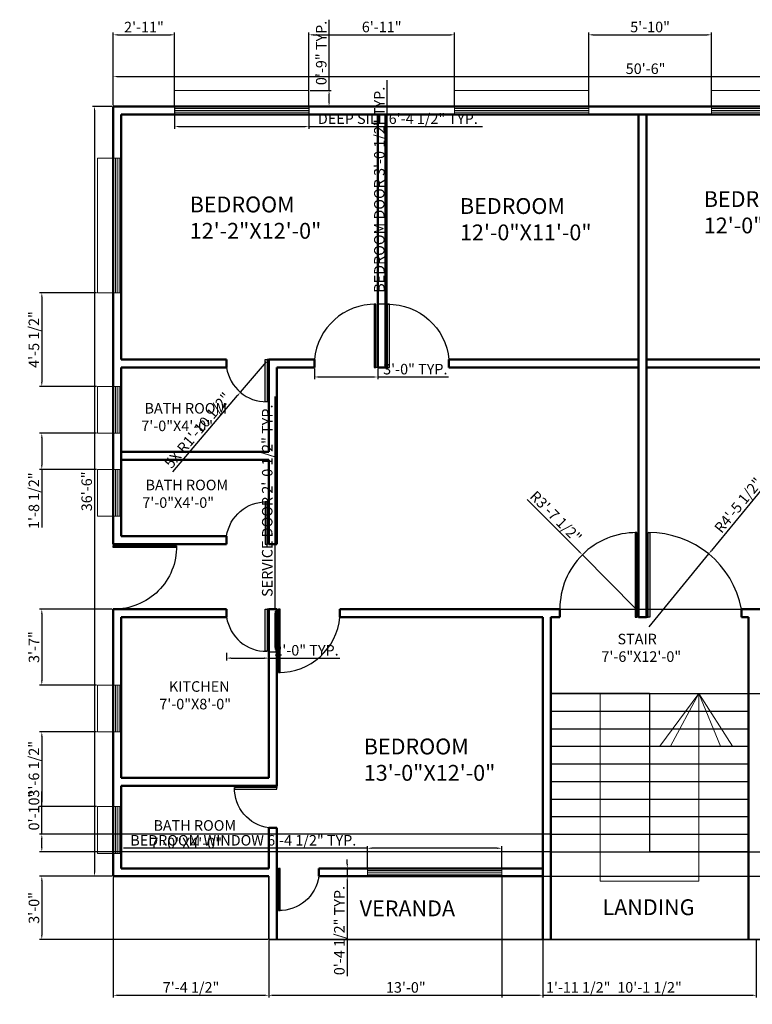
# Model space of a CAD drawing. Units: inches. Extents: x 2373 to 3112, y 1710 to 2270.
# Tile 1 of 2: x 2373 to 2790, y 1710 to 2270. Entities that reach past the tile are written whole.
import ezdxf

# ---------------------------------------------------------------- set-up
doc = ezdxf.new("R2010")
doc.units = ezdxf.units.IN
doc.layers.add('A-ANNO-DIMS', color=7, linetype='Continuous', lineweight=18)
doc.layers.add('A-AREA-IDEN', color=7, linetype='Continuous', lineweight=25)
for name, color, linetype, lineweight, true_color in [('A-ANNO-SYMB', 12, 'Continuous', 18, 0xbc0111), ('A-DOOR', 114, 'Continuous', 25, 0x139b48), ('A-FLOR', 114, 'Continuous', 35, 0x139b48), ('A-FLOR-STRS', 114, 'Continuous', 25, 0x139b48), ('A-GLAZ', 31, 'Continuous', 18, 0xfecc66), ('A-GLAZ-SILL', 30, 'Continuous', 18, 0xf8991e), ('A-WALL', 114, 'Continuous', 50, 0x139b48)]:
    doc.layers.add(name, color=color, linetype=linetype, lineweight=lineweight, true_color=true_color)
doc.styles.get("Standard").update_dxf_attribs({"font": 'arial.ttf'})
doc.dimstyles.new('ISO-25', dxfattribs={"dimtxt": 6, "dimasz": 2.5, "dimexe": 1.25, "dimexo": 0.625, "dimtad": 1, "dimdec": 1, "dimlunit": 3, "dimtxsty": 'Standard', "dimcen": 2.5, "dimadec": 0, "dimazin": 0, "dimtfac": 1, "dimtdec": 1, "dimtmove": 0, "dimatfit": 3, "dimfxl": 1, "dimarcsym": 0})

# ---------------------------------------------------------------- blocks, each defined once
blk = doc.blocks.new('*D2')
at = {"layer": 'A-ANNO-DIMS', "color": 0, "lineweight": -2, "transparency": 16777216}
for p, q in [((2426.36, 2221.72), (2426.36, 2239.32)), ((2428.86, 2238.07), (3029.86, 2238.07)), ((3032.36, 2221.72), (3032.36, 2239.32))]:
    blk.add_line(p, q, dxfattribs=at)
at = {"layer": 'A-ANNO-DIMS', "color": 0, "transparency": 16777216}
for points in [[(2428.86, 2238.48), (2428.86, 2237.65), (2426.36, 2238.07)], [(3029.86, 2238.48), (3029.86, 2237.65), (3032.36, 2238.07)]]:
    blk.add_solid(points, dxfattribs=at)
at = {"layer": 'Defpoints', "color": 0, "transparency": 16777216}
for p in [(3032.36, 2238.07), (2426.36, 2221.09), (3032.36, 2221.09)]:
    blk.add_point(p, dxfattribs=at)
at = {"layer": 'A-ANNO-DIMS', "color": 0, "transparency": 16777216, "insert": (2729.36, 2241.76), "char_height": 6, "attachment_point": 5}
blk.add_mtext('50\'-6"', dxfattribs=at)
blk = doc.blocks.new('*D3')
at = {"layer": 'A-ANNO-DIMS', "color": 0, "lineweight": -2, "transparency": 16777216}
for p, q in [((2425.74, 2221.09), (2414.44, 2221.09)), ((2415.69, 2218.59), (2415.69, 1785.59)), ((2425.74, 1783.09), (2414.44, 1783.09))]:
    blk.add_line(p, q, dxfattribs=at)
at = {"layer": 'A-ANNO-DIMS', "color": 0, "transparency": 16777216}
for points in [[(2415.27, 2218.59), (2416.11, 2218.59), (2415.69, 2221.09)], [(2415.27, 1785.59), (2416.11, 1785.59), (2415.69, 1783.09)]]:
    blk.add_solid(points, dxfattribs=at)
at = {"layer": 'Defpoints', "color": 0, "transparency": 16777216}
for p in [(2426.36, 2221.09), (2415.69, 1783.09), (2426.36, 1783.09)]:
    blk.add_point(p, dxfattribs=at)
at = {"layer": 'A-ANNO-DIMS', "color": 0, "transparency": 16777216, "insert": (2412, 2002.09), "char_height": 6, "attachment_point": 5, "rotation": 90}
blk.add_mtext('36\'-6"', dxfattribs=at)
blk = doc.blocks.new('DOOR-SWING-24IN')
for p, q in [((-2, -24), (-2, 0)), ((-2, 0), (-1, 0)), ((0, 0), (-1, 0)), ((-1, 0), (-1, -24)), ((-1, -24), (-2, -24))]:
    blk.add_line(p, q)
blk.add_arc((-1.5, -1.28), 22.73, 188.1552, 271.2605)
blk = doc.blocks.new('DOOR-SWING-36IN')
for p, q in [((-1, 36), (-2, 36)), ((-2, 36), (-2, 0)), ((-1, 0), (-1, 36)), ((-2, 0), (-1, 0)), ((0, 0), (-1, 0))]:
    blk.add_line(p, q)
blk.add_arc((-1.5, 1.36), 34.64, 89.173, 174.8014)
blk = doc.blocks.new('DOOR-SIDE-ENTRY-36IN')
for p, q in [((0, 0), (0, -1)), ((0, -1), (-36, -1)), ((-36, -1), (-36, -2)), ((-36, -2), (0, -2)), ((0, -2), (0, -1))]:
    blk.add_line(p, q)
blk.add_arc((-0.5, -1.5), 35.5, 179.1931, 270.8069)
blk = doc.blocks.new('WINDOW-BEDROOM')
for p, q in [((0, 0), (0, -4.5)), ((76.46, 0), (0, 0)), ((0, 0), (0, -2.25)), ((76.46, -4.5), (76.46, 0)), ((76.46, -1.25), (0, -1.25)), ((0, -1.25), (0, -2.25)), ((0, -2.25), (76.46, -2.25)), ((0, -2.25), (0, -3.25)), ((0, -3.25), (76.46, -3.25)), ((0, -4.5), (76.46, -4.5)), ((76.46, -2.25), (76.46, -1.25))]:
    blk.add_line(p, q)
blk = doc.blocks.new('WINDOW-SERVICE')
for p, q in [((0, 0), (0, -26.66)), ((4.5, 0), (0, 0)), ((1.25, 0), (1.25, -26.66)), ((2.25, 0), (2.25, -26.66)), ((3.25, -26.66), (3.25, 0)), ((4.5, -26.66), (4.5, 0)), ((4.5, -26.66), (4.5, 0)), ((0, -26.66), (4.5, -26.66))]:
    blk.add_line(p, q)
blk = doc.blocks.new('SILL-SERVICE')
for p, q in [((0, 0), (9, 0)), ((9, 0), (9, -26.66)), ((9, -26.66), (0, -26.66))]:
    blk.add_line(p, q)
blk = doc.blocks.new('SILL-BEDROOM')
for p, q in [((0, 0), (0, 9)), ((0, 9), (76.46, 9)), ((76.46, 9), (76.46, 0))]:
    blk.add_line(p, q)
blk = doc.blocks.new('SILL-BEDROOM-DEEP')
for p, q in [((0, 0), (0, 9.02)), ((0, 9.02), (76.46, 9.02)), ((76.46, 9.02), (76.46, 0))]:
    blk.add_line(p, q)
blk = doc.blocks.new('*D12')
at = {"layer": 'A-ANNO-DIMS', "color": 0, "lineweight": -2, "transparency": 16777216}
for p, q in [((2518.5, 1935.09), (2518.5, 2055.97)), ((2515.49, 1935.09), (2519.75, 1935.09)), ((2518.5, 1913.34), (2518.5, 1932.59)), ((2515.49, 1910.84), (2519.75, 1910.84))]:
    blk.add_line(p, q, dxfattribs=at)
at = {"layer": 'A-ANNO-DIMS', "color": 0, "transparency": 16777216}
for points in [[(2518.08, 1932.59), (2518.92, 1932.59), (2518.5, 1935.09)], [(2518.08, 1913.34), (2518.92, 1913.34), (2518.5, 1910.84)]]:
    blk.add_solid(points, dxfattribs=at)
at = {"layer": 'Defpoints', "color": 0, "transparency": 16777216}
for p in [(2514.86, 1935.09), (2518.5, 1935.09), (2514.86, 1910.84)]:
    blk.add_point(p, dxfattribs=at)
at = {"layer": 'A-ANNO-DIMS', "color": 0, "transparency": 16777216, "insert": (2514.77, 1996.78), "char_height": 6, "attachment_point": 5, "rotation": 90}
blk.add_mtext('SERVICE DOOR 2\'-0 1/2" TYP.', dxfattribs=at)
blk = doc.blocks.new('*D13')
at = {"layer": 'A-ANNO-DIMS', "color": 0, "lineweight": -2, "transparency": 16777216}
for p, q in [((2490.86, 1910.22), (2490.86, 1905.95)), ((2493.36, 1907.2), (2512.36, 1907.2)), ((2514.86, 1910.22), (2514.86, 1905.95)), ((2514.86, 1907.2), (2555.29, 1907.2))]:
    blk.add_line(p, q, dxfattribs=at)
at = {"layer": 'A-ANNO-DIMS', "color": 0, "transparency": 16777216}
for points in [[(2493.36, 1907.62), (2493.36, 1906.79), (2490.86, 1907.2)], [(2512.36, 1907.62), (2512.36, 1906.79), (2514.86, 1907.2)]]:
    blk.add_solid(points, dxfattribs=at)
at = {"layer": 'Defpoints', "color": 0, "transparency": 16777216}
for p in [(2490.86, 1910.84), (2514.86, 1910.84), (2514.86, 1907.2)]:
    blk.add_point(p, dxfattribs=at)
at = {"layer": 'A-ANNO-DIMS', "color": 0, "transparency": 16777216, "insert": (2536.33, 1910.89), "char_height": 6, "attachment_point": 5}
blk.add_mtext('2\'-0" TYP.', dxfattribs=at)
blk = doc.blocks.new('*D14')
at = {"layer": 'A-ANNO-DIMS', "color": 0, "lineweight": -2, "transparency": 16777216}
for p, q in [((2582.3, 2108.86), (2582.3, 2236.01)), ((2577.49, 2108.86), (2583.55, 2108.86)), ((2582.3, 2075.09), (2582.3, 2106.36)), ((2577.49, 2072.59), (2583.55, 2072.59))]:
    blk.add_line(p, q, dxfattribs=at)
at = {"layer": 'A-ANNO-DIMS', "color": 0, "transparency": 16777216}
for points in [[(2581.89, 2106.36), (2582.72, 2106.36), (2582.3, 2108.86)], [(2581.89, 2075.09), (2582.72, 2075.09), (2582.3, 2072.59)]]:
    blk.add_solid(points, dxfattribs=at)
at = {"layer": 'Defpoints', "color": 0, "transparency": 16777216}
for p in [(2576.86, 2108.86), (2582.3, 2108.86), (2576.86, 2072.59)]:
    blk.add_point(p, dxfattribs=at)
at = {"layer": 'A-ANNO-DIMS', "color": 0, "transparency": 16777216, "insert": (2578.57, 2173.68), "char_height": 6, "attachment_point": 5, "rotation": 90}
blk.add_mtext('BEDROOM DOOR 3\'-0 1/2" TYP.', dxfattribs=at)
blk = doc.blocks.new('*D15')
at = {"layer": 'A-ANNO-DIMS', "color": 0, "lineweight": -2, "transparency": 16777216}
for p, q in [((2540.86, 2071.97), (2540.86, 2065.91)), ((2543.36, 2067.16), (2574.36, 2067.16)), ((2576.86, 2071.97), (2576.86, 2065.91)), ((2576.86, 2067.16), (2617.18, 2067.16))]:
    blk.add_line(p, q, dxfattribs=at)
at = {"layer": 'A-ANNO-DIMS', "color": 0, "transparency": 16777216}
for points in [[(2543.36, 2067.57), (2543.36, 2066.74), (2540.86, 2067.16)], [(2574.36, 2067.57), (2574.36, 2066.74), (2576.86, 2067.16)]]:
    blk.add_solid(points, dxfattribs=at)
at = {"layer": 'Defpoints', "color": 0, "transparency": 16777216}
for p in [(2540.86, 2072.59), (2576.86, 2072.59), (2576.86, 2067.16)]:
    blk.add_point(p, dxfattribs=at)
at = {"layer": 'A-ANNO-DIMS', "color": 0, "transparency": 16777216, "insert": (2598.27, 2070.85), "char_height": 6, "attachment_point": 5}
blk.add_mtext('3\'-0" TYP.', dxfattribs=at)
blk = doc.blocks.new('*D18')
at = {"layer": 'A-ANNO-DIMS', "color": 0, "lineweight": -2, "transparency": 16777216}
for p, q in [((2571, 1799.06), (2432.22, 1799.06)), ((2571, 1788.22), (2571, 1800.31)), ((2644.96, 1799.06), (2573.5, 1799.06)), ((2647.46, 1788.22), (2647.46, 1800.31))]:
    blk.add_line(p, q, dxfattribs=at)
at = {"layer": 'A-ANNO-DIMS', "color": 0, "transparency": 16777216}
for points in [[(2573.5, 1799.48), (2573.5, 1798.65), (2571, 1799.06)], [(2644.96, 1799.48), (2644.96, 1798.65), (2647.46, 1799.06)]]:
    blk.add_solid(points, dxfattribs=at)
at = {"layer": 'Defpoints', "color": 0, "transparency": 16777216}
for p in [(2571, 1799.06), (2571, 1787.59), (2647.46, 1787.59)]:
    blk.add_point(p, dxfattribs=at)
at = {"layer": 'A-ANNO-DIMS', "color": 0, "transparency": 16777216, "insert": (2500.36, 1802.79), "char_height": 6, "attachment_point": 5}
blk.add_mtext('BEDROOM WINDOW 6\'-4 1/2" TYP.', dxfattribs=at)
blk = doc.blocks.new('*D19')
at = {"layer": 'A-ANNO-DIMS', "color": 0, "lineweight": -2, "transparency": 16777216}
for p, q in [((2559.53, 1790.09), (2559.53, 1792.59)), ((2570.38, 1787.59), (2558.28, 1787.59)), ((2559.53, 1787.59), (2559.53, 1783.09)), ((2570.38, 1783.09), (2558.28, 1783.09)), ((2559.53, 1780.59), (2559.53, 1726.29))]:
    blk.add_line(p, q, dxfattribs=at)
at = {"layer": 'A-ANNO-DIMS', "color": 0, "transparency": 16777216}
for points in [[(2559.12, 1790.09), (2559.95, 1790.09), (2559.53, 1787.59)], [(2559.12, 1780.59), (2559.95, 1780.59), (2559.53, 1783.09)]]:
    blk.add_solid(points, dxfattribs=at)
at = {"layer": 'Defpoints', "color": 0, "transparency": 16777216}
for p in [(2571, 1787.59), (2559.53, 1783.09), (2571, 1783.09)]:
    blk.add_point(p, dxfattribs=at)
at = {"layer": 'A-ANNO-DIMS', "color": 0, "transparency": 16777216, "insert": (2555.81, 1752.19), "char_height": 6, "attachment_point": 5, "rotation": 90}
blk.add_mtext('0\'-4 1/2" TYP.', dxfattribs=at)
blk = doc.blocks.new('*D26')
at = {"layer": 'A-ANNO-DIMS', "color": 0, "lineweight": -2, "transparency": 16777216}
for p, q in [((2461.26, 2220.47), (2461.26, 2208.38)), ((2537.72, 2220.47), (2537.72, 2208.38)), ((2463.76, 2209.63), (2535.22, 2209.63)), ((2537.72, 2209.63), (2636.45, 2209.63))]:
    blk.add_line(p, q, dxfattribs=at)
at = {"layer": 'A-ANNO-DIMS', "color": 0, "transparency": 16777216}
for points in [[(2463.76, 2210.04), (2463.76, 2209.21), (2461.26, 2209.63)], [(2535.22, 2210.04), (2535.22, 2209.21), (2537.72, 2209.63)]]:
    blk.add_solid(points, dxfattribs=at)
at = {"layer": 'Defpoints', "color": 0, "transparency": 16777216}
for p in [(2461.26, 2221.09), (2537.72, 2221.09), (2537.72, 2209.63)]:
    blk.add_point(p, dxfattribs=at)
at = {"layer": 'A-ANNO-DIMS', "color": 0, "transparency": 16777216, "insert": (2588.34, 2213.35), "char_height": 6, "attachment_point": 5}
blk.add_mtext('DEEP SILL 6\'-4 1/2" TYP.', dxfattribs=at)
blk = doc.blocks.new('*D27')
at = {"layer": 'A-ANNO-DIMS', "color": 0, "lineweight": -2, "transparency": 16777216}
for p, q in [((2549.19, 2230.11), (2549.19, 2270.44)), ((2538.35, 2230.11), (2550.44, 2230.11)), ((2549.19, 2223.59), (2549.19, 2227.61)), ((2538.35, 2221.09), (2550.44, 2221.09))]:
    blk.add_line(p, q, dxfattribs=at)
at = {"layer": 'A-ANNO-DIMS', "color": 0, "transparency": 16777216}
for points in [[(2548.77, 2227.61), (2549.61, 2227.61), (2549.19, 2230.11)], [(2548.77, 2223.59), (2549.61, 2223.59), (2549.19, 2221.09)]]:
    blk.add_solid(points, dxfattribs=at)
at = {"layer": 'Defpoints', "color": 0, "transparency": 16777216}
for p in [(2537.72, 2230.11), (2549.19, 2230.11), (2537.72, 2221.09)]:
    blk.add_point(p, dxfattribs=at)
at = {"layer": 'A-ANNO-DIMS', "color": 0, "transparency": 16777216, "insert": (2545.5, 2251.52), "char_height": 6, "attachment_point": 5, "rotation": 90}
blk.add_mtext('0\'-9" TYP.', dxfattribs=at)
blk = doc.blocks.new('*D28')
at = {"layer": 'A-ANNO-DIMS', "color": 0, "lineweight": -2, "transparency": 16777216}
for p, q in [((2425.74, 1783.09), (2384.41, 1783.09)), ((2385.66, 1780.59), (2385.66, 1749.59)), ((2514.24, 1747.09), (2384.41, 1747.09))]:
    blk.add_line(p, q, dxfattribs=at)
at = {"layer": 'A-ANNO-DIMS', "color": 0, "transparency": 16777216}
for points in [[(2385.24, 1780.59), (2386.08, 1780.59), (2385.66, 1783.09)], [(2385.24, 1749.59), (2386.08, 1749.59), (2385.66, 1747.09)]]:
    blk.add_solid(points, dxfattribs=at)
at = {"layer": 'Defpoints', "color": 0, "transparency": 16777216}
for p in [(2426.36, 1783.09), (2385.66, 1747.09), (2514.86, 1747.09)]:
    blk.add_point(p, dxfattribs=at)
at = {"layer": 'A-ANNO-DIMS', "color": 0, "transparency": 16777216, "insert": (2381.97, 1765.09), "char_height": 6, "attachment_point": 5, "rotation": 90}
blk.add_mtext('3\'-0"', dxfattribs=at)
blk = doc.blocks.new('*D29')
at = {"layer": 'A-ANNO-DIMS', "color": 0, "lineweight": -2, "transparency": 16777216}
for p, q in [((2426.36, 1782.47), (2426.36, 1714.14)), ((2514.86, 1746.47), (2514.86, 1714.14)), ((2428.86, 1715.39), (2512.36, 1715.39))]:
    blk.add_line(p, q, dxfattribs=at)
at = {"layer": 'A-ANNO-DIMS', "color": 0, "transparency": 16777216}
for points in [[(2428.86, 1715.81), (2428.86, 1714.97), (2426.36, 1715.39)], [(2512.36, 1715.81), (2512.36, 1714.97), (2514.86, 1715.39)]]:
    blk.add_solid(points, dxfattribs=at)
at = {"layer": 'Defpoints', "color": 0, "transparency": 16777216}
for p in [(2426.36, 1783.09), (2514.86, 1747.09), (2514.86, 1715.39)]:
    blk.add_point(p, dxfattribs=at)
at = {"layer": 'A-ANNO-DIMS', "color": 0, "transparency": 16777216, "insert": (2470.61, 1719.12), "char_height": 6, "attachment_point": 5}
blk.add_mtext('7\'-4 1/2"', dxfattribs=at)
blk = doc.blocks.new('*D30')
at = {"layer": 'A-ANNO-DIMS', "color": 0, "lineweight": -2, "transparency": 16777216}
for p, q in [((2514.86, 1746.47), (2514.86, 1714.14)), ((2670.86, 1746.47), (2670.86, 1714.14)), ((2517.36, 1715.39), (2668.36, 1715.39))]:
    blk.add_line(p, q, dxfattribs=at)
at = {"layer": 'A-ANNO-DIMS', "color": 0, "transparency": 16777216}
for points in [[(2517.36, 1715.81), (2517.36, 1714.97), (2514.86, 1715.39)], [(2668.36, 1715.81), (2668.36, 1714.97), (2670.86, 1715.39)]]:
    blk.add_solid(points, dxfattribs=at)
at = {"layer": 'Defpoints', "color": 0, "transparency": 16777216}
for p in [(2514.86, 1747.09), (2670.86, 1747.09), (2670.86, 1715.39)]:
    blk.add_point(p, dxfattribs=at)
at = {"layer": 'A-ANNO-DIMS', "color": 0, "transparency": 16777216, "insert": (2592.86, 1719.08), "char_height": 6, "attachment_point": 5}
blk.add_mtext('13\'-0"', dxfattribs=at)
blk = doc.blocks.new('*D31')
at = {"layer": 'A-ANNO-DIMS', "color": 0, "lineweight": -2, "transparency": 16777216}
for p, q in [((2670.86, 1746.47), (2670.86, 1714.14)), ((2792.36, 1746.47), (2792.36, 1714.14)), ((2673.36, 1715.39), (2789.86, 1715.39))]:
    blk.add_line(p, q, dxfattribs=at)
at = {"layer": 'A-ANNO-DIMS', "color": 0, "transparency": 16777216}
for points in [[(2673.36, 1715.81), (2673.36, 1714.97), (2670.86, 1715.39)], [(2789.86, 1715.81), (2789.86, 1714.97), (2792.36, 1715.39)]]:
    blk.add_solid(points, dxfattribs=at)
at = {"layer": 'Defpoints', "color": 0, "transparency": 16777216}
for p in [(2670.86, 1747.09), (2792.36, 1747.09), (2792.36, 1715.39)]:
    blk.add_point(p, dxfattribs=at)
at = {"layer": 'A-ANNO-DIMS', "color": 0, "transparency": 16777216, "insert": (2731.61, 1719.12), "char_height": 6, "attachment_point": 5}
blk.add_mtext('10\'-1 1/2"', dxfattribs=at)
blk = doc.blocks.new('*D34')
at = {"layer": 'A-ANNO-DIMS', "color": 0, "lineweight": -2, "transparency": 16777216}
for p, q in [((2555.99, 1935.09), (3074.32, 1935.09)), ((3073.07, 1785.59), (3073.07, 1932.59)), ((2571.63, 1783.09), (3074.32, 1783.09))]:
    blk.add_line(p, q, dxfattribs=at)
at = {"layer": 'A-ANNO-DIMS', "color": 0, "transparency": 16777216}
for points in [[(3072.65, 1932.59), (3073.49, 1932.59), (3073.07, 1935.09)], [(3072.65, 1785.59), (3073.49, 1785.59), (3073.07, 1783.09)]]:
    blk.add_solid(points, dxfattribs=at)
at = {"layer": 'Defpoints', "color": 0, "transparency": 16777216}
for p in [(2555.36, 1935.09), (3073.07, 1935.09), (2571, 1783.09)]:
    blk.add_point(p, dxfattribs=at)
at = {"layer": 'A-ANNO-DIMS', "color": 0, "transparency": 16777216, "insert": (3069.38, 1859.09), "char_height": 6, "attachment_point": 5, "rotation": 90}
blk.add_mtext('12\'-8"', dxfattribs=at)
blk = doc.blocks.new('*D35')
at = {"layer": 'A-ANNO-DIMS', "color": 0, "lineweight": -2, "transparency": 16777216}
for p, q in [((2426.36, 2221.72), (2426.36, 2263.07)), ((2428.86, 2261.82), (2458.76, 2261.82)), ((2461.26, 2221.72), (2461.26, 2263.07))]:
    blk.add_line(p, q, dxfattribs=at)
at = {"layer": 'A-ANNO-DIMS', "color": 0, "transparency": 16777216}
for points in [[(2428.86, 2262.24), (2428.86, 2261.4), (2426.36, 2261.82)], [(2458.76, 2262.24), (2458.76, 2261.4), (2461.26, 2261.82)]]:
    blk.add_solid(points, dxfattribs=at)
at = {"layer": 'Defpoints', "color": 0, "transparency": 16777216}
for p in [(2461.26, 2261.82), (2426.36, 2221.09), (2461.26, 2221.09)]:
    blk.add_point(p, dxfattribs=at)
at = {"layer": 'A-ANNO-DIMS', "color": 0, "transparency": 16777216, "insert": (2443.81, 2265.46), "char_height": 6, "attachment_point": 5}
blk.add_mtext('2\'-11"', dxfattribs=at)
blk = doc.blocks.new('*D36')
at = {"layer": 'A-ANNO-DIMS', "color": 0, "lineweight": -2, "transparency": 16777216}
for p, q in [((2537.72, 2221.72), (2537.72, 2263.07)), ((2540.22, 2261.82), (2618.05, 2261.82)), ((2620.55, 2221.72), (2620.55, 2263.07))]:
    blk.add_line(p, q, dxfattribs=at)
at = {"layer": 'A-ANNO-DIMS', "color": 0, "transparency": 16777216}
for points in [[(2540.22, 2262.24), (2540.22, 2261.4), (2537.72, 2261.82)], [(2618.05, 2262.24), (2618.05, 2261.4), (2620.55, 2261.82)]]:
    blk.add_solid(points, dxfattribs=at)
at = {"layer": 'Defpoints', "color": 0, "transparency": 16777216}
for p in [(2620.55, 2261.82), (2537.72, 2221.09), (2620.55, 2221.09)]:
    blk.add_point(p, dxfattribs=at)
at = {"layer": 'A-ANNO-DIMS', "color": 0, "transparency": 16777216, "insert": (2579.14, 2265.51), "char_height": 6, "attachment_point": 5}
blk.add_mtext('6\'-11"', dxfattribs=at)
blk = doc.blocks.new('*D37')
at = {"layer": 'A-ANNO-DIMS', "color": 0, "lineweight": -2, "transparency": 16777216}
for p, q in [((2697.01, 2221.72), (2697.01, 2263.07)), ((2699.51, 2261.82), (2764.3, 2261.82)), ((2766.8, 2221.72), (2766.8, 2263.07))]:
    blk.add_line(p, q, dxfattribs=at)
at = {"layer": 'A-ANNO-DIMS', "color": 0, "transparency": 16777216}
for points in [[(2699.51, 2262.24), (2699.51, 2261.4), (2697.01, 2261.82)], [(2764.3, 2262.24), (2764.3, 2261.4), (2766.8, 2261.82)]]:
    blk.add_solid(points, dxfattribs=at)
at = {"layer": 'Defpoints', "color": 0, "transparency": 16777216}
for p in [(2766.8, 2261.82), (2697.01, 2221.09), (2766.8, 2221.09)]:
    blk.add_point(p, dxfattribs=at)
at = {"layer": 'A-ANNO-DIMS', "color": 0, "transparency": 16777216, "insert": (2731.91, 2265.51), "char_height": 6, "attachment_point": 5}
blk.add_mtext('5\'-10"', dxfattribs=at)
blk = doc.blocks.new('*D45')
at = {"layer": 'A-ANNO-DIMS', "color": 0, "lineweight": -2, "transparency": 16777216}
for p, q in [((2416.74, 2115.12), (2384.41, 2115.12)), ((2385.66, 2112.62), (2385.66, 2064.33)), ((2416.74, 2061.83), (2384.41, 2061.83))]:
    blk.add_line(p, q, dxfattribs=at)
at = {"layer": 'A-ANNO-DIMS', "color": 0, "transparency": 16777216}
for points in [[(2385.24, 2112.62), (2386.08, 2112.62), (2385.66, 2115.12)], [(2385.24, 2064.33), (2386.08, 2064.33), (2385.66, 2061.83)]]:
    blk.add_solid(points, dxfattribs=at)
at = {"layer": 'Defpoints', "color": 0, "transparency": 16777216}
for p in [(2417.36, 2115.12), (2385.66, 2061.83), (2417.36, 2061.83)]:
    blk.add_point(p, dxfattribs=at)
at = {"layer": 'A-ANNO-DIMS', "color": 0, "transparency": 16777216, "insert": (2381.93, 2088.47), "char_height": 6, "attachment_point": 5, "rotation": 90}
blk.add_mtext('4\'-5 1/2"', dxfattribs=at)
blk = doc.blocks.new('*D46')
at = {"layer": 'A-ANNO-DIMS', "color": 0, "lineweight": -2, "transparency": 16777216}
for p, q in [((2416.74, 2035.17), (2384.41, 2035.17)), ((2385.66, 2032.67), (2385.66, 2017.08)), ((2416.74, 2014.58), (2384.41, 2014.58)), ((2385.66, 2014.58), (2385.66, 1981.47))]:
    blk.add_line(p, q, dxfattribs=at)
at = {"layer": 'A-ANNO-DIMS', "color": 0, "transparency": 16777216}
for points in [[(2385.24, 2032.67), (2386.08, 2032.67), (2385.66, 2035.17)], [(2385.24, 2017.08), (2386.08, 2017.08), (2385.66, 2014.58)]]:
    blk.add_solid(points, dxfattribs=at)
at = {"layer": 'Defpoints', "color": 0, "transparency": 16777216}
for p in [(2417.36, 2035.17), (2385.66, 2014.58), (2417.36, 2014.58)]:
    blk.add_point(p, dxfattribs=at)
at = {"layer": 'A-ANNO-DIMS', "color": 0, "transparency": 16777216, "insert": (2381.93, 1996.78), "char_height": 6, "attachment_point": 5, "rotation": 90}
blk.add_mtext('1\'-8 1/2"', dxfattribs=at)
blk = doc.blocks.new('*D47')
at = {"layer": 'A-ANNO-DIMS', "color": 0, "lineweight": -2, "transparency": 16777216}
for p, q in [((2425.74, 1935.09), (2384.41, 1935.09)), ((2385.66, 1932.59), (2385.66, 1894.38)), ((2416.74, 1891.88), (2384.41, 1891.88))]:
    blk.add_line(p, q, dxfattribs=at)
at = {"layer": 'A-ANNO-DIMS', "color": 0, "transparency": 16777216}
for points in [[(2385.24, 1932.59), (2386.08, 1932.59), (2385.66, 1935.09)], [(2385.24, 1894.38), (2386.08, 1894.38), (2385.66, 1891.88)]]:
    blk.add_solid(points, dxfattribs=at)
at = {"layer": 'Defpoints', "color": 0, "transparency": 16777216}
for p in [(2426.36, 1935.09), (2385.66, 1891.88), (2417.36, 1891.88)]:
    blk.add_point(p, dxfattribs=at)
at = {"layer": 'A-ANNO-DIMS', "color": 0, "transparency": 16777216, "insert": (2381.97, 1913.49), "char_height": 6, "attachment_point": 5, "rotation": 90}
blk.add_mtext('3\'-7"', dxfattribs=at)
blk = doc.blocks.new('*D48')
at = {"layer": 'A-ANNO-DIMS', "color": 0, "lineweight": -2, "transparency": 16777216}
for p, q in [((2416.74, 1865.22), (2384.41, 1865.22)), ((2385.66, 1862.72), (2385.66, 1825.25)), ((2416.74, 1822.75), (2384.41, 1822.75))]:
    blk.add_line(p, q, dxfattribs=at)
at = {"layer": 'A-ANNO-DIMS', "color": 0, "transparency": 16777216}
for points in [[(2385.24, 1862.72), (2386.08, 1862.72), (2385.66, 1865.22)], [(2385.24, 1825.25), (2386.08, 1825.25), (2385.66, 1822.75)]]:
    blk.add_solid(points, dxfattribs=at)
at = {"layer": 'Defpoints', "color": 0, "transparency": 16777216}
for p in [(2417.36, 1865.22), (2385.66, 1822.75), (2417.36, 1822.75)]:
    blk.add_point(p, dxfattribs=at)
at = {"layer": 'A-ANNO-DIMS', "color": 0, "transparency": 16777216, "insert": (2381.93, 1843.98), "char_height": 6, "attachment_point": 5, "rotation": 90}
blk.add_mtext('3\'-6 1/2"', dxfattribs=at)
blk = doc.blocks.new('*D50')
at = {"layer": 'A-ANNO-DIMS', "color": 0, "lineweight": -2, "transparency": 16777216}
for p, q in [((2647.46, 1782.47), (2647.46, 1714.14)), ((2670.86, 1782.47), (2670.86, 1714.14)), ((2649.96, 1715.39), (2668.36, 1715.39)), ((2670.86, 1715.39), (2708.64, 1715.39))]:
    blk.add_line(p, q, dxfattribs=at)
at = {"layer": 'A-ANNO-DIMS', "color": 0, "transparency": 16777216}
for points in [[(2649.96, 1715.81), (2649.96, 1714.97), (2647.46, 1715.39)], [(2668.36, 1715.81), (2668.36, 1714.97), (2670.86, 1715.39)]]:
    blk.add_solid(points, dxfattribs=at)
at = {"layer": 'Defpoints', "color": 0, "transparency": 16777216}
for p in [(2647.46, 1783.09), (2670.86, 1783.09), (2670.86, 1715.39)]:
    blk.add_point(p, dxfattribs=at)
at = {"layer": 'A-ANNO-DIMS', "color": 0, "transparency": 16777216, "insert": (2691, 1719.12), "char_height": 6, "attachment_point": 5}
blk.add_mtext('1\'-11 1/2"', dxfattribs=at)
blk = doc.blocks.new('*D51')
at = {"layer": 'A-ANNO-DIMS', "color": 0, "lineweight": -2, "transparency": 16777216}
for p, q in [((2385.66, 1807.04), (2385.66, 1831.41)), ((2674.74, 1807.04), (2384.41, 1807.04)), ((2385.66, 1799.54), (2385.66, 1804.54)), ((2674.74, 1797.04), (2384.41, 1797.04))]:
    blk.add_line(p, q, dxfattribs=at)
at = {"layer": 'A-ANNO-DIMS', "color": 0, "transparency": 16777216}
for points in [[(2385.24, 1804.54), (2386.08, 1804.54), (2385.66, 1807.04)], [(2385.24, 1799.54), (2386.08, 1799.54), (2385.66, 1797.04)]]:
    blk.add_solid(points, dxfattribs=at)
at = {"layer": 'Defpoints', "color": 0, "transparency": 16777216}
for p in [(2385.66, 1807.04), (2675.36, 1807.04), (2675.36, 1797.04)]:
    blk.add_point(p, dxfattribs=at)
at = {"layer": 'A-ANNO-DIMS', "color": 0, "transparency": 16777216, "insert": (2381.97, 1820.47), "char_height": 6, "attachment_point": 5, "rotation": 90}
blk.add_mtext('0\'-10"', dxfattribs=at)
blk = doc.blocks.new('*D52')
at = {"layer": 'A-ANNO-DIMS', "color": 0, "lineweight": -2, "transparency": 16777216}
for p, q in [((2788.49, 1887.04), (3074.32, 1887.04)), ((3073.07, 1799.54), (3073.07, 1884.54)), ((2788.49, 1797.04), (3074.32, 1797.04))]:
    blk.add_line(p, q, dxfattribs=at)
at = {"layer": 'A-ANNO-DIMS', "color": 0, "transparency": 16777216}
for points in [[(3072.65, 1884.54), (3073.49, 1884.54), (3073.07, 1887.04)], [(3072.65, 1799.54), (3073.49, 1799.54), (3073.07, 1797.04)]]:
    blk.add_solid(points, dxfattribs=at)
at = {"layer": 'Defpoints', "color": 0, "transparency": 16777216}
for p in [(2787.86, 1887.04), (3073.07, 1887.04), (2787.86, 1797.04)]:
    blk.add_point(p, dxfattribs=at)
at = {"layer": 'A-ANNO-DIMS', "color": 0, "transparency": 16777216, "insert": (3069.38, 1842.04), "char_height": 6, "attachment_point": 5, "rotation": 90}
blk.add_mtext('7\'-6"', dxfattribs=at)
blk = doc.blocks.new('*D53')
at = {"layer": 'A-ANNO-DIMS', "color": 0, "lineweight": -2, "transparency": 16777216}
for p, q in [((2797.34, 2005.57), (2766.87, 1968.4)), ((2731.36, 1925.09), (2765.28, 1966.47))]:
    blk.add_line(p, q, dxfattribs=at)
at = {"layer": 'A-ANNO-DIMS', "color": 0, "transparency": 16777216}
blk.add_solid([(2766.55, 1968.67), (2767.19, 1968.14), (2765.28, 1966.47)], dxfattribs=at)
at = {"layer": 'Defpoints', "color": 0, "transparency": 16777216}
for p in [(2765.28, 1966.47), (2731.36, 1925.09)]:
    blk.add_point(p, dxfattribs=at)
at = {"layer": 'A-ANNO-DIMS', "color": 0, "transparency": 16777216, "insert": (2782.75, 1993.66), "char_height": 6, "attachment_point": 5, "rotation": 50.654}
blk.add_mtext('R4\'-5 1/2"', dxfattribs=at)
blk = doc.blocks.new('*D54')
at = {"layer": 'A-ANNO-DIMS', "color": 0, "lineweight": -2, "transparency": 16777216}
for p, q in [((2662.04, 1997.53), (2691.6, 1967.79)), ((2723.86, 1935.32), (2693.36, 1966.02))]:
    blk.add_line(p, q, dxfattribs=at)
at = {"layer": 'A-ANNO-DIMS', "color": 0, "transparency": 16777216}
blk.add_solid([(2691.89, 1968.09), (2691.3, 1967.5), (2693.36, 1966.02)], dxfattribs=at)
at = {"layer": 'Defpoints', "color": 0, "transparency": 16777216}
for p in [(2693.36, 1966.02), (2723.86, 1935.32)]:
    blk.add_point(p, dxfattribs=at)
at = {"layer": 'A-ANNO-DIMS', "color": 0, "transparency": 16777216, "insert": (2677.7, 1987.07), "char_height": 6, "attachment_point": 5, "rotation": 314.8187}
blk.add_mtext('R3\'-7 1/2"', dxfattribs=at)
blk = doc.blocks.new('*D57')
at = {"layer": 'A-ANNO-DIMS', "color": 0, "lineweight": -2, "transparency": 16777216}
for p, q in [((2513.36, 2075.82), (2498.66, 2058.48)), ((2460.2, 2013.12), (2497.05, 2056.58))]:
    blk.add_line(p, q, dxfattribs=at)
at = {"layer": 'A-ANNO-DIMS', "color": 0, "transparency": 16777216}
blk.add_solid([(2496.73, 2056.84), (2497.37, 2056.31), (2498.66, 2058.48)], dxfattribs=at)
at = {"layer": 'Defpoints', "color": 0, "transparency": 16777216}
for p in [(2513.36, 2075.82), (2498.66, 2058.48)]:
    blk.add_point(p, dxfattribs=at)
at = {"layer": 'A-ANNO-DIMS', "color": 0, "transparency": 16777216, "insert": (2474.97, 2036.3), "char_height": 6, "attachment_point": 5, "rotation": 49.7064}
blk.add_mtext('5X R1\'-10 1/2"', dxfattribs=at)

msp = doc.modelspace()

# ---------------------------------------------------------------- linework, layer by layer
at = {"layer": 'A-ANNO-SYMB'}
for p, q in [((2703.49, 1887.04), (2703.49, 1780.28)), ((2759.74, 1887.04), (2737.54, 1857.04)), ((2759.74, 1887.04), (2743.62, 1857.04)), ((2743.62, 1857.04), (2759.74, 1887.04)), ((2759.74, 1780.28), (2759.74, 1887.04)), ((2759.74, 1887.04), (2771.92, 1857.04)), ((2759.74, 1887.04), (2778.76, 1857.04)), ((2759.74, 1797.04), (2759.74, 1780.28)), ((2703.49, 1780.28), (2759.74, 1780.28))]:
    msp.add_line(p, q, dxfattribs=at)
at = {"layer": 'A-DOOR'}
for p, q in [((2724.36, 1978.59), (2723.36, 1978.59)), ((2723.36, 1978.59), (2723.36, 1930.59)), ((2724.36, 1930.59), (2724.36, 1978.59)), ((2730.86, 1930.59), (2730.86, 1978.59)), ((2730.86, 1978.59), (2731.86, 1978.59)), ((2731.86, 1978.59), (2731.86, 1930.59)), ((2723.36, 1930.59), (2724.36, 1930.59)), ((2725.36, 1930.59), (2724.36, 1930.59)), ((2729.86, 1930.59), (2730.86, 1930.59)), ((2731.86, 1930.59), (2730.86, 1930.59))]:
    msp.add_line(p, q, dxfattribs=at)
for centre, radius, start, end in [((2723.86, 1935.32), 43.28, 89.338, 180.2996), ((2731.36, 1925.09), 53.5, 10.7721, 90.5355)]:
    msp.add_arc(centre, radius, start, end, dxfattribs=at)
at = {"layer": 'A-FLOR'}
for p, q in [((2514.86, 1783.09), (2514.86, 1747.09)), ((2514.86, 1747.09), (2948.36, 1747.09))]:
    msp.add_line(p, q, dxfattribs=at)
at = {"layer": 'A-FLOR-STRS'}
for p, q in [((2675.36, 1887.04), (2787.86, 1887.04)), ((2731.61, 1887.04), (2675.36, 1887.04)), ((2675.36, 1887.04), (2703.49, 1887.04)), ((2731.61, 1887.04), (2731.61, 1797.04)), ((2675.36, 1877.04), (2787.86, 1877.04)), ((2675.36, 1867.04), (2787.86, 1867.04)), ((2675.36, 1857.04), (2787.86, 1857.04)), ((2675.36, 1847.04), (2787.86, 1847.04)), ((2675.36, 1837.04), (2787.86, 1837.04)), ((2675.36, 1827.04), (2787.86, 1827.04)), ((2675.36, 1817.04), (2787.86, 1817.04)), ((2675.36, 1807.04), (2787.86, 1807.04)), ((2675.36, 1797.04), (2787.86, 1797.04)), ((2787.86, 1797.04), (2731.61, 1797.04)), ((2731.61, 1797.04), (2759.74, 1797.04))]:
    msp.add_line(p, q, dxfattribs=at)
at = {"layer": 'A-WALL'}
for p, q in [((2426.36, 2221.09), (3032.36, 2221.09)), ((2426.36, 1972.09), (2426.36, 2221.09)), ((2430.86, 2216.59), (3027.86, 2216.59)), ((2430.86, 2077.09), (2430.86, 2216.59)), ((2576.86, 2072.59), (2576.86, 2216.59)), ((2581.36, 2072.59), (2581.36, 2216.59)), ((2725.36, 1930.59), (2725.36, 2216.59)), ((2729.86, 1930.59), (2729.86, 2216.59)), ((2430.86, 2077.09), (2490.86, 2077.09)), ((2490.86, 2077.09), (2490.86, 2072.59)), ((2514.86, 2072.59), (2514.86, 2077.09)), ((2514.86, 2077.09), (2540.86, 2077.09)), ((2540.86, 2072.59), (2540.86, 2077.09)), ((2617.36, 2072.59), (2617.36, 2077.09)), ((2617.36, 2077.09), (2725.36, 2077.09)), ((2729.86, 2077.09), (2841.36, 2077.09)), ((2430.86, 2072.59), (2490.86, 2072.59)), ((2430.86, 1976.59), (2430.86, 2072.59)), ((2514.86, 2024.59), (2514.86, 2072.59)), ((2519.36, 2072.59), (2540.86, 2072.59)), ((2519.36, 1972.09), (2519.36, 2072.59)), ((2576.86, 2072.59), (2581.36, 2072.59)), ((2617.36, 2072.59), (2725.36, 2072.59)), ((2729.86, 2072.59), (2841.36, 2072.59)), ((2430.86, 2024.59), (2514.86, 2024.59)), ((2430.86, 2020.09), (2514.86, 2020.09)), ((2514.86, 1972.09), (2514.86, 2020.09)), ((2426.36, 1972.09), (2490.86, 1972.09)), ((2430.86, 1976.59), (2490.86, 1976.59)), ((2490.86, 1976.59), (2490.86, 1972.09)), ((2514.86, 1976.59), (2514.86, 1972.09)), ((2514.86, 1972.09), (2519.36, 1972.09)), ((2426.36, 1783.09), (2426.36, 1935.09)), ((2426.36, 1935.09), (2490.86, 1935.09)), ((2490.86, 1930.59), (2490.86, 1935.09)), ((2514.86, 1935.09), (2519.36, 1935.09)), ((2514.86, 1839.09), (2514.86, 1935.09)), ((2519.36, 1834.59), (2519.36, 1935.09)), ((2555.36, 1935.09), (2555.36, 1930.59)), ((2555.36, 1935.09), (2680.59, 1935.09)), ((2680.59, 1935.09), (2680.59, 1930.59)), ((2783.92, 1935.09), (2783.92, 1930.59)), ((2783.92, 1935.09), (2907.86, 1935.09)), ((2430.86, 1930.59), (2490.86, 1930.59)), ((2430.86, 1839.09), (2430.86, 1930.59)), ((2555.36, 1930.59), (2670.86, 1930.59)), ((2670.86, 1747.09), (2670.86, 1930.59)), ((2675.36, 1747.09), (2675.36, 1930.59)), ((2675.36, 1930.59), (2680.59, 1930.59)), ((2725.36, 1930.59), (2729.86, 1930.59)), ((2783.92, 1930.59), (2787.86, 1930.59)), ((2787.86, 1930.59), (2787.86, 1747.09)), ((2430.86, 1839.09), (2514.86, 1839.09)), ((2430.86, 1787.59), (2430.86, 1834.59)), ((2430.86, 1834.59), (2519.36, 1834.59)), ((2514.86, 1787.59), (2514.86, 1810.59)), ((2519.36, 1810.59), (2514.86, 1810.59)), ((2519.36, 1747.09), (2519.36, 1810.59)), ((2514.86, 1787.59), (2430.86, 1787.59)), ((2670.86, 1787.59), (2543.36, 1787.59)), ((2543.36, 1783.09), (2543.36, 1787.59)), ((2514.86, 1783.09), (2426.36, 1783.09)), ((2670.86, 1783.09), (2543.36, 1783.09))]:
    msp.add_line(p, q, dxfattribs=at)

# ---------------------------------------------------------------- block references
at = {"layer": 'A-DOOR'}
for name, p in [('DOOR-SWING-36IN', (2576.86, 2072.59)), ('DOOR-SWING-24IN', (2514.86, 2077.09)), ('DOOR-SWING-24IN', (2514.86, 1935.09))]:
    msp.add_blockref(name, p, dxfattribs=at)
at = {"layer": 'A-DOOR', "extrusion": (0, 0, -1), "zscale": -1}
for name, p in [('DOOR-SWING-36IN', (-2581.36, 2072.59)), ('DOOR-SIDE-ENTRY-36IN', (-2426.36, 1972.09)), ('DOOR-SWING-24IN', (-2519.36, 1787.59))]:
    msp.add_blockref(name, p, dxfattribs=at)
for p, rotation in [((-2514.86, 1972.09), 180), ((-2519.36, 1834.59), 90.00000000000644)]:
    msp.add_blockref('DOOR-SWING-24IN', p, dxfattribs=dict(at, rotation=rotation))
at = {"layer": 'A-DOOR', "rotation": 180}
msp.add_blockref('DOOR-SWING-36IN', (2519.36, 1935.09), dxfattribs=at)
at = {"layer": 'A-GLAZ'}
for name, p in [('WINDOW-BEDROOM', (2461.26, 2221.09)), ('WINDOW-BEDROOM', (2620.55, 2221.09)), ('WINDOW-BEDROOM', (2766.8, 2221.09)), ('WINDOW-SERVICE', (2426.36, 2061.83)), ('WINDOW-SERVICE', (2426.36, 2014.58)), ('WINDOW-SERVICE', (2426.36, 1891.88)), ('WINDOW-SERVICE', (2426.36, 1822.75))]:
    msp.add_blockref(name, p, dxfattribs=at)
for p, rotation in [((2426.36, 2115.12), 90.0000000000012), ((2647.46, 1783.09), 180)]:
    msp.add_blockref('WINDOW-BEDROOM', p, dxfattribs=dict(at, rotation=rotation))
at = {"layer": 'A-GLAZ-SILL'}
for name, p in [('SILL-BEDROOM-DEEP', (2461.26, 2221.09)), ('SILL-BEDROOM-DEEP', (2620.55, 2221.09)), ('SILL-BEDROOM', (2766.8, 2221.09))]:
    msp.add_blockref(name, p, dxfattribs=at)
for name, p, rotation in [('SILL-BEDROOM', (2426.36, 2115.12), 89.99999999999834), ('SILL-SERVICE', (2426.36, 2035.17), 180), ('SILL-SERVICE', (2426.36, 1987.93), 180), ('SILL-SERVICE', (2426.36, 1865.22), 180), ('SILL-SERVICE', (2426.36, 1796.09), 180)]:
    msp.add_blockref(name, p, dxfattribs=dict(at, rotation=rotation))

# ---------------------------------------------------------------- texts
at = {"layer": 'A-AREA-IDEN', "attachment_point": 1}
for s, insert, char_height in [('BEDROOM\\P12\'-2"X12\'-0"', (2469.85, 2169.82), 9), ('BEDROOM\\P12\'-0"X11\'-0"', (2623.69, 2168.92), 9), ('BEDROOM\\P12\'-0"X11\'-0"', (2762.49, 2172.87), 9), (' BATH ROOM\\P   7\'-0"X4\'-0"', (2442.29, 2052.34), 6), (' BATH ROOM\\P   7\'-0"X4\'-0"', (2442.86, 2008.7), 6), ('     STAIR\\P   7\'-6"X12\'-0"', (2704.21, 1921.08), 6), ('   KITCHEN\\P   7\'-0"X8\'-0"', (2452.54, 1894.06), 6), ('BEDROOM\\P13\'-0"X12\'-0"', (2568.94, 1861.44), 9), (' BATH ROOM\\P   7\'-0"X4\'-0"', (2447.38, 1815.02), 6), ('VERANDA', (2566.56, 1769.35), 9)]:
    msp.add_mtext(s, dxfattribs=dict(at, insert=insert, char_height=char_height))
at = {"layer": 'A-AREA-IDEN', "insert": (2704.8, 1769.98), "char_height": 9, "width": 60.7469, "attachment_point": 1}
msp.add_mtext('LANDING', dxfattribs=at)

# ---------------------------------------------------------------- dimensions: what is measured, and where the dimension line sits
at = {"layer": 'A-ANNO-DIMS'}
for base, p1, p2, override, picture, middle in [((2461.26, 2261.82), (2426.36, 2221.09), (2461.26, 2221.09), {"dimdec": 1, "dimlfac": 1, "dimrnd": 0, "dimzin": 1, "dimdsep": 46, "dimlunit": 4, "dimfrac": 2}, '*D35', (2443.81, 2265.46)), ((2620.55, 2261.82), (2537.72, 2221.09), (2620.55, 2221.09), {"dimdec": 1, "dimlfac": 1, "dimrnd": 0, "dimzin": 1, "dimdsep": 46, "dimlunit": 4, "dimfrac": 2}, '*D36', (2579.14, 2265.51)), ((2766.8, 2261.82), (2697.01, 2221.09), (2766.8, 2221.09), {"dimdec": 1, "dimlfac": 1, "dimrnd": 0, "dimzin": 1, "dimdsep": 46, "dimlunit": 4, "dimfrac": 2}, '*D37', (2731.91, 2265.51)), ((3032.36, 2238.07), (2426.36, 2221.09), (3032.36, 2221.09), {"dimclrd": 0, "dimclre": 0, "dimclrt": 0}, '*D2', (2729.36, 2241.76)), ((2514.86, 1715.39), (2426.36, 1783.09), (2514.86, 1747.09), {"dimdec": 1, "dimlfac": 1, "dimrnd": 0, "dimzin": 1, "dimdsep": 46, "dimlunit": 4, "dimfrac": 2}, '*D29', (2470.61, 1719.12)), ((2670.86, 1715.39), (2647.46, 1783.09), (2670.86, 1783.09), {"dimdec": 1, "dimlfac": 1, "dimrnd": 0, "dimzin": 1, "dimdsep": 46, "dimlunit": 4, "dimfrac": 2}, '*D50', (2691, 1719.12)), ((2670.86, 1715.39), (2514.86, 1747.09), (2670.86, 1747.09), {"dimdec": 1, "dimlfac": 1, "dimrnd": 0, "dimzin": 1, "dimdsep": 46, "dimlunit": 4, "dimfrac": 2}, '*D30', (2592.86, 1719.08)), ((2792.36, 1715.39), (2670.86, 1747.09), (2792.36, 1747.09), {"dimdec": 1, "dimlfac": 1, "dimrnd": 0, "dimzin": 1, "dimdsep": 46, "dimlunit": 4, "dimfrac": 2}, '*D31', (2731.61, 1719.12))]:
    dim = msp.add_linear_dim(base=base, p1=p1, p2=p2, dimstyle='ISO-25', override=override, dxfattribs=at)
    dim.commit()
    dim.dimension.update_dxf_attribs({"geometry": picture, "text_midpoint": middle})
for base, p1, p2, angle, text, picture, middle in [((2549.19, 2230.11), (2537.72, 2221.09), (2537.72, 2230.11), 90, '<> TYP.', '*D27', (2545.5, 2251.52)), ((2582.3, 2108.86), (2576.86, 2072.59), (2576.86, 2108.86), 90, 'BEDROOM DOOR <> TYP.', '*D14', (2578.57, 2173.68)), ((2518.5014, 1935.0946), (2514.8635, 1910.8417), (2514.8635, 1935.0946), 90, 'SERVICE DOOR <> TYP.', '*D12', (2514.7721, 1996.783)), ((2571, 1799.06), (2647.46, 1787.59), (2571, 1787.59), 180, 'BEDROOM WINDOW <> TYP.', '*D18', (2500.36, 1802.79)), ((2559.53, 1783.09), (2571, 1787.59), (2571, 1783.09), 270, '<> TYP.', '*D19', (2555.81, 1752.19))]:
    dim = msp.add_linear_dim(base=base, p1=p1, p2=p2, angle=angle, text=text, dimstyle='ISO-25', override={"dimdec": 1, "dimlfac": 1, "dimrnd": 0, "dimzin": 1, "dimdsep": 46, "dimlunit": 4, "dimfrac": 2}, dxfattribs=at)
    dim.commit()
    dim.dimension.update_dxf_attribs({"geometry": picture, "text_midpoint": middle})
for base, p1, p2, text, picture, middle in [((2537.72, 2209.63), (2461.26, 2221.09), (2537.72, 2221.09), 'DEEP SILL <> TYP.', '*D26', (2588.34, 2213.35)), ((2576.86, 2067.16), (2540.86, 2072.59), (2576.86, 2072.59), '<> TYP.', '*D15', (2598.27, 2070.85)), ((2514.86, 1907.2), (2490.86, 1910.84), (2514.86, 1910.84), '<> TYP.', '*D13', (2536.33, 1910.89))]:
    dim = msp.add_linear_dim(base=base, p1=p1, p2=p2, text=text, dimstyle='ISO-25', override={"dimdec": 1, "dimlfac": 1, "dimrnd": 0, "dimzin": 1, "dimdsep": 46, "dimlunit": 4, "dimfrac": 2}, dxfattribs=at)
    dim.commit()
    dim.dimension.update_dxf_attribs({"geometry": picture, "text_midpoint": middle})
for base, p1, p2, override, picture, middle in [((2415.69, 1783.09), (2426.36, 2221.09), (2426.36, 1783.09), {"dimclrd": 0, "dimclre": 0, "dimclrt": 0}, '*D3', (2412, 2002.09)), ((2385.66, 2061.83), (2417.36, 2115.12), (2417.36, 2061.83), {"dimdec": 1, "dimlfac": 1, "dimrnd": 0, "dimzin": 1, "dimdsep": 46, "dimlunit": 4, "dimfrac": 2}, '*D45', (2381.93, 2088.47)), ((2385.66, 2014.58), (2417.36, 2035.17), (2417.36, 2014.58), {"dimdec": 1, "dimlfac": 1, "dimrnd": 0, "dimzin": 1, "dimdsep": 46, "dimlunit": 4, "dimfrac": 2}, '*D46', (2381.93, 1996.78)), ((2385.66, 1891.88), (2426.36, 1935.09), (2417.36, 1891.88), {"dimdec": 1, "dimlfac": 1, "dimrnd": 0, "dimzin": 1, "dimdsep": 46, "dimlunit": 4, "dimfrac": 2}, '*D47', (2381.97, 1913.49)), ((3073.07, 1935.09), (2571, 1783.09), (2555.36, 1935.09), {"dimdec": 1, "dimlfac": 1, "dimrnd": 0, "dimzin": 1, "dimdsep": 46, "dimlunit": 4, "dimfrac": 2}, '*D34', (3069.38, 1859.09)), ((3073.07, 1887.04), (2787.86, 1797.04), (2787.86, 1887.04), {"dimdec": 1, "dimlfac": 1, "dimrnd": 0, "dimzin": 1, "dimdsep": 46, "dimlunit": 4, "dimfrac": 2}, '*D52', (3069.38, 1842.04)), ((2385.66, 1822.75), (2417.36, 1865.22), (2417.36, 1822.75), {"dimdec": 1, "dimlfac": 1, "dimrnd": 0, "dimzin": 1, "dimdsep": 46, "dimlunit": 4, "dimfrac": 2}, '*D48', (2381.93, 1843.98)), ((2385.66, 1807.04), (2675.36, 1797.04), (2675.36, 1807.04), {"dimdec": 1, "dimlfac": 1, "dimrnd": 0, "dimzin": 1, "dimdsep": 46, "dimlunit": 4, "dimfrac": 2}, '*D51', (2381.97, 1820.47)), ((2385.66, 1747.09), (2426.36, 1783.09), (2514.86, 1747.09), {"dimdec": 1, "dimlfac": 1, "dimrnd": 0, "dimzin": 1, "dimdsep": 46, "dimlunit": 4, "dimfrac": 2}, '*D28', (2381.97, 1765.09))]:
    dim = msp.add_linear_dim(base=base, p1=p1, p2=p2, angle=90, dimstyle='ISO-25', override=override, dxfattribs=at)
    dim.commit()
    dim.dimension.update_dxf_attribs({"geometry": picture, "text_midpoint": middle})
dim = msp.add_radius_dim(center=(2513.36, 2075.82), mpoint=(2498.66, 2058.48), text='5X <>', dimstyle='ISO-25', override={"dimdec": 1, "dimlfac": 1, "dimrnd": 0, "dimzin": 1, "dimdsep": 46, "dimlunit": 4, "dimfrac": 2}, dxfattribs=at)
dim.commit()
dim.dimension.update_dxf_attribs({"geometry": '*D57', "text_midpoint": (2474.97, 2036.3)})
for center, mpoint, picture, middle in [((2731.36, 1925.09), (2765.28, 1966.47), '*D53', (2785.64, 1991.29)), ((2723.86, 1935.32), (2693.36, 1966.02), '*D54', (2675.06, 1984.44))]:
    dim = msp.add_radius_dim(center=center, mpoint=mpoint, dimstyle='ISO-25', override={"dimdec": 1, "dimlfac": 1, "dimrnd": 0, "dimzin": 1, "dimdsep": 46, "dimlunit": 4, "dimfrac": 2}, dxfattribs=at)
    dim.commit()
    dim.dimension.update_dxf_attribs({"geometry": picture, "text_midpoint": middle, "dimtype": 164})

doc.saveas('drawing.dxf')
